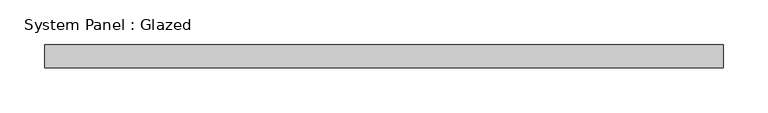
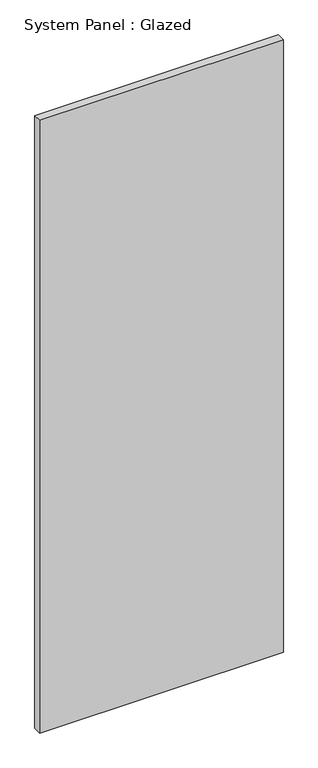
"""IFC4 building model written with IfcOpenShell, lengths in millimetres: plate geometry, System Panel : Glazed."""

from ifc_helpers import new_model, si_unit, origin, origin_with_axes, place, context, project, spatial, polyline, outline, extrude, source, transform, mapped, element, save


def system_panel_glazed_a3b3c321(model_context):
    return source(origin(), model_context, "Body", "SweptSolid", [
        extrude(outline(polyline([(377.825, -44.45), (-377.825, -44.45), (-377.825, -19.05), (377.825, -19.05), (377.825, -44.45)])), origin_with_axes(), (0.0, 0.0, 1.0), 2006.6),
    ])


if __name__ == "__main__":
    model = new_model("IFC4")
    model_context = context("Model", 3, world=origin())
    ifc_project = project(units=[si_unit("LENGTHUNIT", "METRE", prefix="MILLI")], contexts=[model_context])
    site = spatial("IfcSite", under=ifc_project)
    building = spatial("IfcBuilding", under=site)
    placement = place(None, origin())
    system_panel_glazed_shape = system_panel_glazed_a3b3c321(model_context)
    element("IfcPlate", 1, ObjectType="System Panel : Glazed", at=placement, inside=building, context=model_context, shape_type="MappedRepresentation", body=[
        mapped(system_panel_glazed_shape, transform((0.0, 0.0, 0.0), x_axis=(1.0, 0.0, 0.0), y_axis=(0.0, 1.0, 0.0), z_axis=(0.0, 0.0, 1.0))),
    ])
    save(model, "model.ifc")

# Revit data of these elements
# Type "System Panel : Glazed"
#   Construction Type Id = "GSP4R"
#   Analytic Construction = "1/8 in Pilkington single glazing"
#   Visual Light Transmittance = 0.9
#   Solar Heat Gain Coefficient = 0.86
#   Heat Transfer Coefficient (U) = 1.18115 BTU/(h·ft²·°F)
#   Define Thermal Properties by = 1
# Element 1 (IfcPlate, "System Panel : Glazed")
#   Materials on its faces: "Glass"
# Materials
#   "Glass": class "Glass", colour RGB 0 128 192, transparency 0.75, Description = "Soda Lime Glass", Cost = 0
